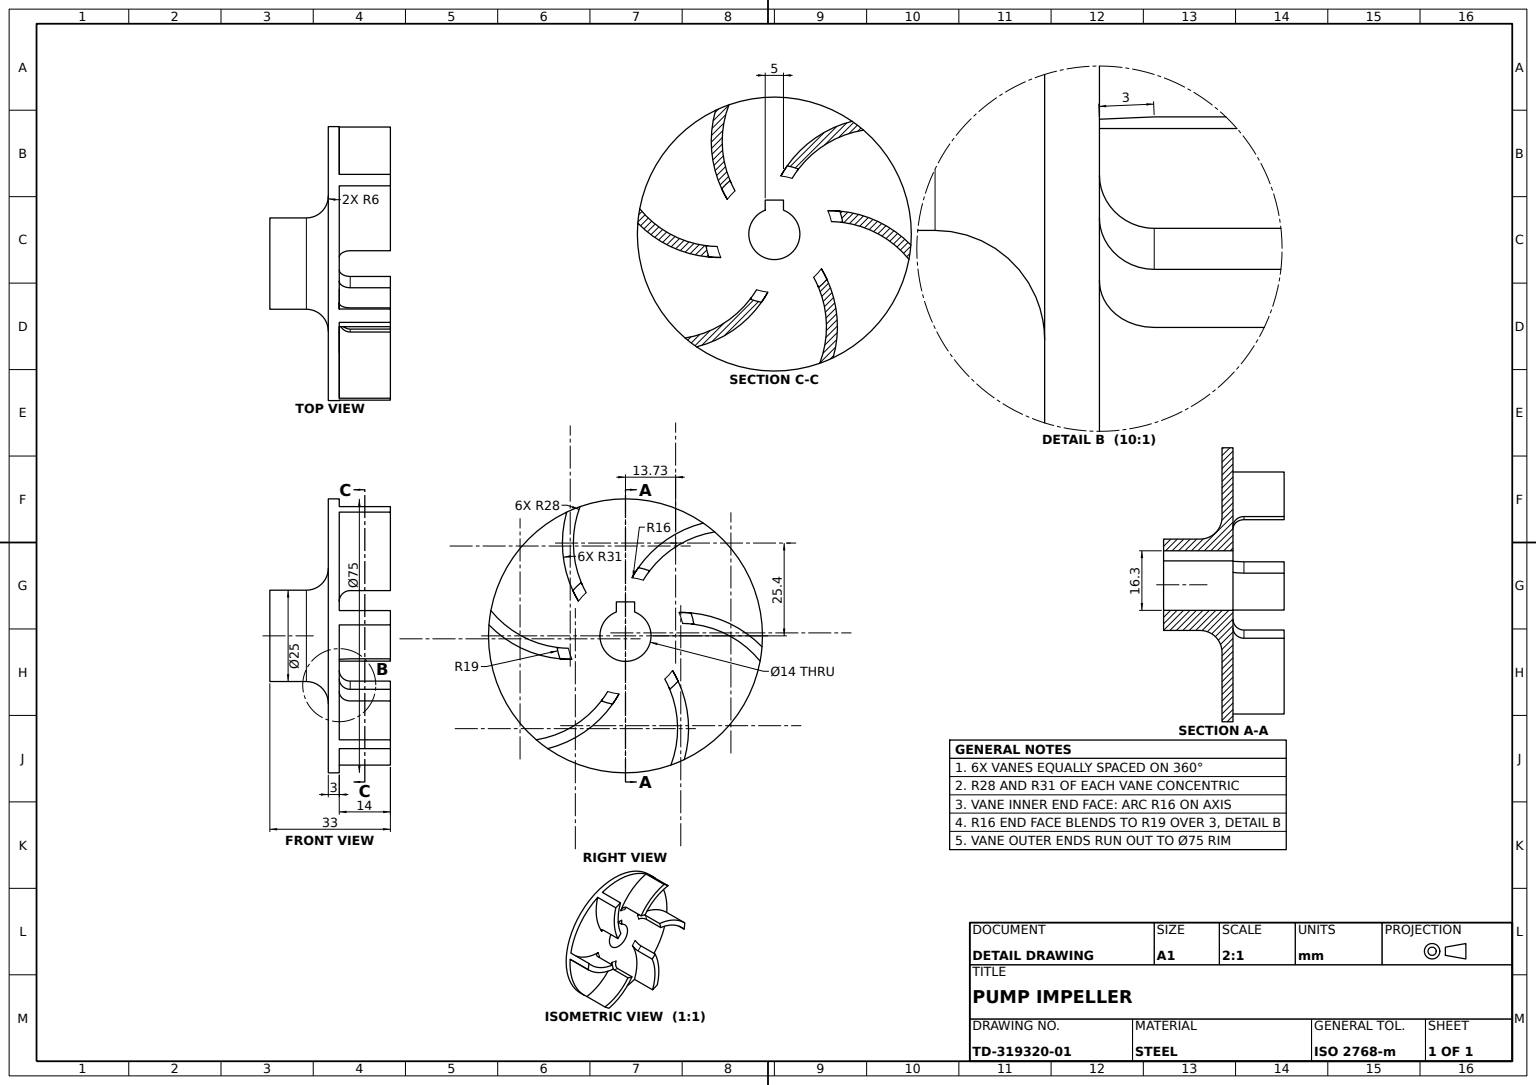
SolidWorks part; units mm, degrees
material "Plain Carbon Steel"
ref_plane "Front Plane" through (0, 0, 0) normal (0, 0, 1) x (1, 0, 0)
ref_plane "Top Plane" through (0, 0, 0) normal (0, 1, 0) x (1, 0, 0)
ref_plane "Right Plane" through (0, 0, 0) normal (1, 0, 0) x (0, 0, -1)
sketch "Back Disc Sketch" plane through (0, 0, 0) normal (0, 0, 1) x (1, 0, 0)
  line L1 (-2.5, 9.3) -> (2.5, 9.3)
  line L2 (-2.5, 9.3) -> (-2.5, 6.5383)
  line L4 (2.5, 9.3) -> (2.5, 6.5383)
  circle A0 centre (0, 0) radius 37.5
  arc A1 (-2.5, 6.5383) -> (2.5, 6.5383) centre (0, 0) ccw
  point P4 (0, 7)
  dimension "D1" = 75
  dimension "D2" = 14
  dimension "D3" = 2.3
  dimension "D4" = 5
extrude "Back Disc Ø75" add sketch "Back Disc Sketch" along normal blind 3
sketch "Hub Sketch" plane through (0, 0, 0) normal (0, 0, -1) x (-1, 0, 0)
  circle A0 centre (0, 0) radius 12.5
  dimension "D1" = 25
extrude "Hub Ø25" add sketch "Hub Sketch" along normal blind 16
sketch "Shaft Bore Sketch" plane through (0, 0, 0) normal (0, 0, 1) x (1, 0, 0)
  line L0 (-2.5, 9.3) -> (-2.5, 6.5383) construction
  line L1 (2.5, 9.3) -> (-2.5, 9.3) construction
  line L2 (2.5, 6.5383) -> (2.5, 9.3) construction
  line L3 (-2.5, 9.3) -> (-2.5, 6.5383)
  line L4 (2.5, 9.3) -> (-2.5, 9.3)
  line L5 (2.5, 6.5383) -> (2.5, 9.3)
  arc A0 (-2.5, 6.5383) -> (2.5, 6.5383) centre (0, 0) ccw construction
  arc A1 (-2.5, 6.5383) -> (2.5, 6.5383) centre (0, 0) ccw
extrude "Shaft Bore" cut sketch "Shaft Bore Sketch" against normal blind 16 contours A1 L5 L4 L3
fillet "Hub Root Fillet R6" radius 6 1 edges at (12.5, 0, 0)
sketch "Vane Sketch" plane through (0, 0, 3) normal (0, 0, 1) x (1, 0, 0)
  line L0 (0, 0) -> (-37.5, 0) construction
  line L1 (-2.5, 9.3) -> (-2.5, 6.5383) construction
  circle A0 centre (0, 0) radius 37.5 construction
  arc A1 (-36.8556, 6.9218) -> (-18.7322, -3.1789) centre (-15.1329, 24.5888) ccw
  arc A2 (-37.3798, 3) -> (-17.9305, -6.2847) centre (-15.1329, 24.5888) ccw
  arc A3 (-36.8556, 6.9218) -> (-37.3798, 3) centre (0, 0) ccw
  arc A4 (-18.7322, -3.1789) -> (-17.9305, -6.2847) centre (0, 0) ccw
  dimension "D3" = 28
  dimension "D4" = 31
  dimension "D1" = 38
  dimension "D2" = 12.6329
  dimension "D5" = 15.4305
extrude "Vane" add sketch "Vane Sketch" along normal blind 14 contours A3 A2 A4 A1
pattern_circular "Vane Pattern 6x" count 6 over 360 about axis through (0, 0, 0) along (0, 0, 1) of "Vane"
fillet "Vane Fillets R3" radius 3 6 edges at (-18.397, -4.7488, 3) (-5.086, -18.3066, 3) (13.311, -13.5579, 3) (18.397, 4.7488, 3) (5.086, 18.3066, 3) (-13.311, 13.5579, 3)
